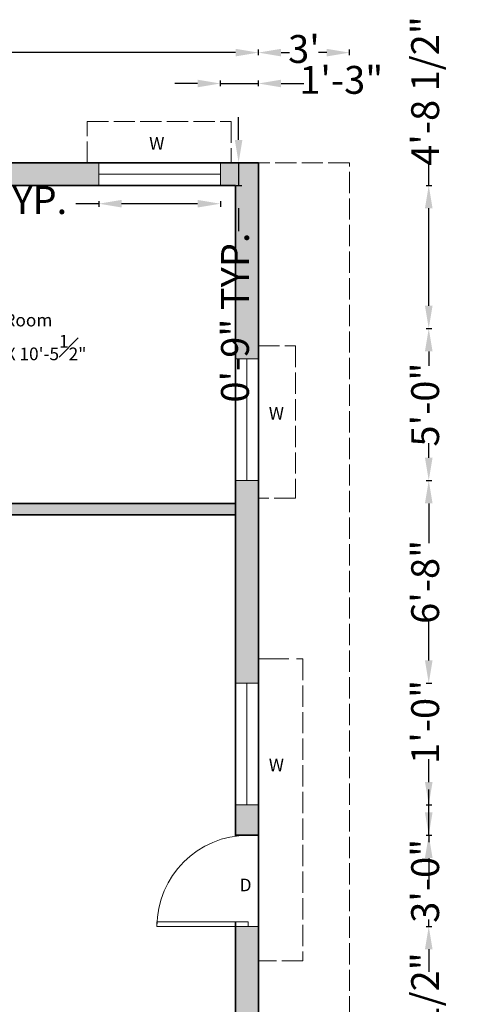
# Model space of a CAD drawing. Units: inches. Extents: x 2339 to 2848, y 489 to 1121.
# Tile 3 of 3: x 2670 to 2848, y 725 to 1114. Entities that reach past the tile are written whole.
import ezdxf

# ---------------------------------------------------------------- set-up
doc = ezdxf.new("R2010")
doc.units = ezdxf.units.IN
doc.linetypes.add('ACAD_ISO02W100', pattern=[15, 12, -3])
for name, color, linetype, lineweight in [('A-ANNO-DIMS', 2, 'Continuous', 18), ('A-ANNO-TEXT', 7, 'Continuous', 18), ('A-AREA-IDEN', 7, 'Continuous', 18), ('A-DOOR', 3, 'Continuous', 18), ('A-GLAZ', 4, 'Continuous', 18), ('A-ROOF-OVHD', 8, 'ACAD_ISO02W100', 13), ('A-WALL', 7, 'Continuous', 35), ('C-PROP', 8, 'ACAD_ISO02W100', 18)]:
    doc.layers.add(name, color=color, linetype=linetype, lineweight=lineweight)
doc.layers.add('A-WALL-PATT', color=18, linetype='Continuous', lineweight=13, true_color=0x000000)
doc.styles.get("Standard").update_dxf_attribs({"font": 'arial.ttf'})
doc.dimstyles.new('ISO-25', dxfattribs={"dimtxt": 11, "dimasz": 9, "dimexe": 1.25, "dimexo": 0.625, "dimtad": 0, "dimlunit": 4, "dimtxsty": 'Standard', "dimcen": 2.5, "dimadec": 0, "dimazin": 0, "dimtfac": 1, "dimtmove": 0, "dimatfit": 3, "dimfxl": 1, "dimfxlon": 1, "dimfrac": 1, "dimarcsym": 0})

# ---------------------------------------------------------------- blocks, each defined once
blk = doc.blocks.new('*U2')
for p, q in [((0, 0), (0, -4)), ((36, 0), (36, -4))]:
    blk.add_line(p, q)
blk.add_lwpolyline([(0, 0), (0, 36), (1.75, 36), (1.75, 0)], close=True)
blk.add_arc((0, 0), 36, 0, 90)
blk = doc.blocks.new('*D6')
at = {"layer": 'A-ANNO-DIMS', "color": 0, "lineweight": -2, "transparency": 16777216}
for p, q in [((2402.35, 1099.88), (2402.35, 1102.13)), ((2411.35, 1100.88), (2563.83, 1100.88)), ((2755.35, 1100.88), (2602.86, 1100.88)), ((2764.35, 1099.88), (2764.35, 1102.13))]:
    blk.add_line(p, q, dxfattribs=at)
at = {"layer": 'A-ANNO-DIMS', "color": 0, "transparency": 16777216}
for points in [[(2411.35, 1102.38), (2411.35, 1099.38), (2402.35, 1100.88)], [(2755.35, 1102.38), (2755.35, 1099.38), (2764.35, 1100.88)]]:
    blk.add_solid(points, dxfattribs=at)
at = {"layer": 'Defpoints', "color": 0, "transparency": 16777216}
for p in [(2764.35, 1100.88), (2402.35, 1057.44), (2764.35, 1057.44)]:
    blk.add_point(p, dxfattribs=at)
at = {"layer": 'A-ANNO-DIMS', "color": 0, "transparency": 16777216, "insert": (2583.35, 1100.88), "char_height": 11, "attachment_point": 5}
blk.add_mtext('30\'-2"', dxfattribs=at)
blk = doc.blocks.new('*D7')
at = {"layer": 'A-ANNO-DIMS', "color": 0, "lineweight": -2, "transparency": 16777216}
for p, q in [((2764.35, 1099.88), (2764.35, 1102.13)), ((2773.35, 1100.88), (2776.66, 1100.88)), ((2791.35, 1100.88), (2788.03, 1100.88)), ((2800.35, 1099.88), (2800.35, 1102.13))]:
    blk.add_line(p, q, dxfattribs=at)
at = {"layer": 'A-ANNO-DIMS', "color": 0, "transparency": 16777216}
for points in [[(2773.35, 1102.38), (2773.35, 1099.38), (2764.35, 1100.88)], [(2791.35, 1102.38), (2791.35, 1099.38), (2800.35, 1100.88)]]:
    blk.add_solid(points, dxfattribs=at)
at = {"layer": 'Defpoints', "color": 0, "transparency": 16777216}
for p in [(2800.35, 1100.88), (2764.35, 1057.44), (2800.35, 1057.44)]:
    blk.add_point(p, dxfattribs=at)
at = {"layer": 'A-ANNO-DIMS', "color": 0, "transparency": 16777216, "insert": (2782.35, 1100.88), "char_height": 11, "attachment_point": 5}
blk.add_mtext("3'", dxfattribs=at)
blk = doc.blocks.new('WIN-48IN')
for p, q in [((0, 0), (0, 9)), ((48, 0), (48, 9)), ((0, 4.5), (48, 4.5))]:
    blk.add_line(p, q)
blk = doc.blocks.new('*D9')
at = {"layer": 'A-ANNO-DIMS', "color": 0, "lineweight": -2, "transparency": 16777216}
for p, q in [((2701.35, 1042.24), (2701.35, 1039.99)), ((2749.35, 1042.24), (2749.35, 1039.99)), ((2701.35, 1041.24), (2692.35, 1041.24)), ((2740.35, 1041.24), (2710.35, 1041.24))]:
    blk.add_line(p, q, dxfattribs=at)
at = {"layer": 'A-ANNO-DIMS', "color": 0, "transparency": 16777216}
for points in [[(2710.35, 1042.74), (2710.35, 1039.74), (2701.35, 1041.24)], [(2740.35, 1042.74), (2740.35, 1039.74), (2749.35, 1041.24)]]:
    blk.add_solid(points, dxfattribs=at)
at = {"layer": 'Defpoints', "color": 0, "transparency": 16777216}
for p in [(2701.35, 1048.44), (2749.35, 1048.44), (2701.35, 1041.24)]:
    blk.add_point(p, dxfattribs=at)
at = {"layer": 'A-ANNO-DIMS', "color": 0, "transparency": 16777216, "insert": (2622.12, 1041.24), "char_height": 11, "attachment_point": 5}
blk.add_mtext('WINDOW 4\'-0" TYP.', dxfattribs=at)
blk = doc.blocks.new('*D10')
at = {"layer": 'A-ANNO-DIMS', "color": 0, "lineweight": -2, "transparency": 16777216}
for p, q in [((2756.55, 1066.44), (2756.55, 1075.44)), ((2755.55, 1057.44), (2757.8, 1057.44)), ((2756.55, 1057.44), (2756.55, 1048.44)), ((2755.55, 1048.44), (2757.8, 1048.44)), ((2756.55, 1039.44), (2756.55, 1030.44))]:
    blk.add_line(p, q, dxfattribs=at)
at = {"layer": 'A-ANNO-DIMS', "color": 0, "transparency": 16777216}
for points in [[(2755.05, 1066.44), (2758.05, 1066.44), (2756.55, 1057.44)], [(2755.05, 1039.44), (2758.05, 1039.44), (2756.55, 1048.44)]]:
    blk.add_solid(points, dxfattribs=at)
at = {"layer": 'Defpoints', "color": 0, "transparency": 16777216}
for p in [(2749.35, 1057.44), (2749.35, 1048.44), (2756.55, 1048.44)]:
    blk.add_point(p, dxfattribs=at)
at = {"layer": 'A-ANNO-DIMS', "color": 0, "transparency": 16777216, "insert": (2756.55, 996.29), "char_height": 11, "attachment_point": 5, "rotation": 90}
blk.add_mtext('0\'-9" TYP.', dxfattribs=at)
blk = doc.blocks.new('*D25')
at = {"layer": 'A-ANNO-DIMS', "color": 0, "lineweight": -2, "transparency": 16777216}
for p, q in [((2830.6, 991.94), (2832.85, 991.94)), ((2831.6, 982.94), (2831.6, 977.18)), ((2831.6, 940.94), (2831.6, 946.69)), ((2830.6, 931.94), (2832.85, 931.94))]:
    blk.add_line(p, q, dxfattribs=at)
at = {"layer": 'A-ANNO-DIMS', "color": 0, "transparency": 16777216}
for points in [[(2830.1, 982.94), (2833.1, 982.94), (2831.6, 991.94)], [(2830.1, 940.94), (2833.1, 940.94), (2831.6, 931.94)]]:
    blk.add_solid(points, dxfattribs=at)
at = {"layer": 'Defpoints', "color": 0, "transparency": 16777216}
for p in [(2411.35, 991.94), (2831.6, 991.94), (2411.35, 931.94)]:
    blk.add_point(p, dxfattribs=at)
at = {"layer": 'A-ANNO-DIMS', "color": 0, "transparency": 16777216, "insert": (2831.6, 961.94), "char_height": 11, "attachment_point": 5, "rotation": 90}
blk.add_mtext('5\'-0"', dxfattribs=at)
blk = doc.blocks.new('*D26')
at = {"layer": 'A-ANNO-DIMS', "color": 0, "lineweight": -2, "transparency": 16777216}
for p, q in [((2831.6, 1048.44), (2831.6, 1057.44)), ((2830.6, 1048.44), (2832.85, 1048.44)), ((2831.6, 1000.94), (2831.6, 1039.44)), ((2830.6, 991.94), (2832.85, 991.94))]:
    blk.add_line(p, q, dxfattribs=at)
at = {"layer": 'A-ANNO-DIMS', "color": 0, "transparency": 16777216}
for points in [[(2830.1, 1039.44), (2833.1, 1039.44), (2831.6, 1048.44)], [(2830.1, 1000.94), (2833.1, 1000.94), (2831.6, 991.94)]]:
    blk.add_solid(points, dxfattribs=at)
at = {"layer": 'Defpoints', "color": 0, "transparency": 16777216}
for p in [(2411.35, 1048.44), (2831.6, 1048.44), (2411.35, 991.94)]:
    blk.add_point(p, dxfattribs=at)
at = {"layer": 'A-ANNO-DIMS', "color": 0, "transparency": 16777216, "insert": (2831.6, 1085.72), "char_height": 11, "attachment_point": 5, "rotation": 90}
blk.add_mtext('4\'-8 1/2"', dxfattribs=at)
blk = doc.blocks.new('*D30')
at = {"layer": 'A-ANNO-DIMS', "color": 0, "lineweight": -2, "transparency": 16777216}
for p, q in [((2740.35, 1088.69), (2731.35, 1088.69)), ((2749.35, 1087.69), (2749.35, 1089.94)), ((2749.35, 1088.69), (2764.35, 1088.69)), ((2764.35, 1087.69), (2764.35, 1089.94)), ((2773.35, 1088.69), (2782.35, 1088.69))]:
    blk.add_line(p, q, dxfattribs=at)
at = {"layer": 'A-ANNO-DIMS', "color": 0, "transparency": 16777216}
for points in [[(2740.35, 1090.19), (2740.35, 1087.19), (2749.35, 1088.69)], [(2773.35, 1090.19), (2773.35, 1087.19), (2764.35, 1088.69)]]:
    blk.add_solid(points, dxfattribs=at)
at = {"layer": 'Defpoints', "color": 0, "transparency": 16777216}
for p in [(2764.35, 1088.69), (2749.35, 1057.44), (2764.35, 1057.44)]:
    blk.add_point(p, dxfattribs=at)
at = {"layer": 'A-ANNO-DIMS', "color": 0, "transparency": 16777216, "insert": (2797.07, 1088.69), "char_height": 11, "attachment_point": 5}
blk.add_mtext('1\'-3"', dxfattribs=at)
blk = doc.blocks.new('*D32')
at = {"layer": 'A-ANNO-DIMS', "color": 0, "lineweight": -2, "transparency": 16777216}
for p, q in [((2830.6, 755.94), (2832.85, 755.94)), ((2831.6, 746.94), (2831.6, 744.28)), ((2831.6, 685.44), (2831.6, 688.1)), ((2830.6, 676.44), (2832.85, 676.44))]:
    blk.add_line(p, q, dxfattribs=at)
at = {"layer": 'A-ANNO-DIMS', "color": 0, "transparency": 16777216}
for points in [[(2830.1, 746.94), (2833.1, 746.94), (2831.6, 755.94)], [(2830.1, 685.44), (2833.1, 685.44), (2831.6, 676.44)]]:
    blk.add_solid(points, dxfattribs=at)
at = {"layer": 'Defpoints', "color": 0, "transparency": 16777216}
for p in [(2764.35, 755.94), (2831.6, 755.94), (2764.35, 676.44)]:
    blk.add_point(p, dxfattribs=at)
at = {"layer": 'A-ANNO-DIMS', "color": 0, "transparency": 16777216, "insert": (2831.6, 716.19), "char_height": 11, "attachment_point": 5, "rotation": 90}
blk.add_mtext('6\'-7 1/2"', dxfattribs=at)
blk = doc.blocks.new('*D33')
at = {"layer": 'A-ANNO-DIMS', "color": 0, "lineweight": -2, "transparency": 16777216}
for p, q in [((2831.6, 800.94), (2831.6, 809.94)), ((2830.6, 791.94), (2832.85, 791.94)), ((2831.6, 791.94), (2831.6, 789.18)), ((2831.6, 755.94), (2831.6, 758.7)), ((2830.6, 755.94), (2832.85, 755.94)), ((2831.6, 746.94), (2831.6, 737.94))]:
    blk.add_line(p, q, dxfattribs=at)
at = {"layer": 'A-ANNO-DIMS', "color": 0, "transparency": 16777216}
for points in [[(2830.1, 800.94), (2833.1, 800.94), (2831.6, 791.94)], [(2830.1, 746.94), (2833.1, 746.94), (2831.6, 755.94)]]:
    blk.add_solid(points, dxfattribs=at)
at = {"layer": 'Defpoints', "color": 0, "transparency": 16777216}
for p in [(2764.35, 791.94), (2831.6, 791.94), (2764.35, 755.94)]:
    blk.add_point(p, dxfattribs=at)
at = {"layer": 'A-ANNO-DIMS', "color": 0, "transparency": 16777216, "insert": (2831.6, 773.94), "char_height": 11, "attachment_point": 5, "rotation": 90}
blk.add_mtext('3\'-0"', dxfattribs=at)
blk = doc.blocks.new('*D34')
at = {"layer": 'A-ANNO-DIMS', "color": 0, "lineweight": -2, "transparency": 16777216}
for p, q in [((2831.6, 812.94), (2831.6, 821.94)), ((2830.6, 803.94), (2832.85, 803.94)), ((2831.6, 791.94), (2831.6, 803.94)), ((2830.6, 791.94), (2832.85, 791.94)), ((2831.6, 782.94), (2831.6, 773.94))]:
    blk.add_line(p, q, dxfattribs=at)
at = {"layer": 'A-ANNO-DIMS', "color": 0, "transparency": 16777216}
for points in [[(2830.1, 812.94), (2833.1, 812.94), (2831.6, 803.94)], [(2830.1, 782.94), (2833.1, 782.94), (2831.6, 791.94)]]:
    blk.add_solid(points, dxfattribs=at)
at = {"layer": 'Defpoints', "color": 0, "transparency": 16777216}
for p in [(2764.35, 803.94), (2831.6, 803.94), (2764.35, 791.94)]:
    blk.add_point(p, dxfattribs=at)
at = {"layer": 'A-ANNO-DIMS', "color": 0, "transparency": 16777216, "insert": (2831.6, 836.67), "char_height": 11, "attachment_point": 5, "rotation": 90}
blk.add_mtext('1\'-0"', dxfattribs=at)
blk = doc.blocks.new('*D35')
at = {"layer": 'A-ANNO-DIMS', "color": 0, "lineweight": -2, "transparency": 16777216}
for p, q in [((2830.6, 931.94), (2832.85, 931.94)), ((2831.6, 922.94), (2831.6, 907.21)), ((2831.6, 860.94), (2831.6, 876.66)), ((2830.6, 851.94), (2832.85, 851.94))]:
    blk.add_line(p, q, dxfattribs=at)
at = {"layer": 'A-ANNO-DIMS', "color": 0, "transparency": 16777216}
for points in [[(2830.1, 922.94), (2833.1, 922.94), (2831.6, 931.94)], [(2830.1, 860.94), (2833.1, 860.94), (2831.6, 851.94)]]:
    blk.add_solid(points, dxfattribs=at)
at = {"layer": 'Defpoints', "color": 0, "transparency": 16777216}
for p in [(2764.35, 931.94), (2831.6, 931.94), (2764.35, 851.94)]:
    blk.add_point(p, dxfattribs=at)
at = {"layer": 'A-ANNO-DIMS', "color": 0, "transparency": 16777216, "insert": (2831.6, 891.94), "char_height": 11, "attachment_point": 5, "rotation": 90}
blk.add_mtext('6\'-8"', dxfattribs=at)

msp = doc.modelspace()

# ---------------------------------------------------------------- hatches: boundary and pattern name
at = {"layer": 'A-WALL-PATT'}
h = msp.add_hatch(color=256, dxfattribs=at)
h.dxf.hatch_style = 1
h.paths.add_polyline_path([(2493.847, 1057.438), (2402.347, 1057.438), (2402.347, 991.938), (2411.347, 991.938), (2411.347, 1048.438), (2493.847, 1048.438)])
h.paths.add_polyline_path([(2411.347, 931.938), (2402.347, 931.938), (2402.347, 912.438), (2411.347, 912.438), (2411.347, 918.438)])
h.paths.add_polyline_path([(2411.347, 871.438), (2411.347, 877.438), (2402.347, 877.438), (2402.347, 803.938), (2411.347, 803.938)])
h.paths.add_polyline_path([(2547.847, 871.438), (2411.347, 871.438), (2411.347, 866.938), (2547.847, 866.938)])
h.paths.add_polyline_path([(2447.347, 922.938), (2411.347, 922.938), (2411.347, 918.438), (2447.347, 918.438)])
h.paths.add_polyline_path([(2552.347, 866.938), (2547.847, 866.938), (2547.847, 791.938), (2552.347, 791.938)])
h.paths.add_polyline_path([(2411.347, 755.938), (2402.347, 755.938), (2402.347, 670.438), (2411.347, 670.438)])
h.paths.add_polyline_path([(2552.347, 755.938), (2547.847, 755.938), (2547.847, 746.938), (2411.347, 746.938), (2411.347, 742.438), (2547.847, 742.438), (2547.847, 737.938), (2552.347, 737.938)])
h.paths.add_polyline_path([(2552.347, 701.938), (2547.847, 701.938), (2547.847, 622.438), (2552.347, 622.438)])
h.paths.add_polyline_path([(2581.347, 622.438), (2411.347, 622.438), (2411.347, 634.438), (2402.347, 634.438), (2402.347, 613.438), (2581.347, 613.438)])
h.paths.add_polyline_path([(2695.347, 622.438), (2635.347, 622.438), (2635.347, 613.438), (2695.347, 613.438)])
h.paths.add_polyline_path([(2764.347, 628.438), (2755.347, 628.438), (2755.347, 622.438), (2749.347, 622.438), (2749.347, 613.438), (2764.347, 613.438)])
h.paths.add_polyline_path([(2764.347, 755.938), (2760.347, 755.938), (2755.347, 755.938), (2755.347, 676.438), (2764.347, 676.438)])
h.paths.add_polyline_path([(2764.347, 931.938), (2755.347, 931.938), (2755.347, 851.938), (2764.347, 851.938)])
h.paths.add_polyline_path([(2764.347, 1057.438), (2749.347, 1057.438), (2749.347, 1048.438), (2755.347, 1048.438), (2755.347, 979.938), (2764.347, 979.938)])
h.paths.add_polyline_path([(2701.347, 1057.438), (2594.347, 1057.438), (2594.347, 1048.438), (2604.847, 1048.438), (2701.347, 1048.438)])
h.paths.add_polyline_path([(2558.347, 1057.438), (2541.847, 1057.438), (2541.847, 1048.438), (2552.347, 1048.438), (2558.347, 1048.438)])
h = msp.add_hatch(color=256, dxfattribs=at)
h.dxf.hatch_style = 1
h.paths.add_polyline_path([(2552.347, 1048.438), (2547.847, 1048.438), (2547.847, 967.438), (2551.847, 967.438), (2552.347, 967.438), (2552.347, 971.938), (2563.847, 971.938), (2563.847, 976.438), (2552.347, 976.438)])
h.paths.add_polyline_path([(2604.847, 1048.438), (2600.347, 1048.438), (2600.347, 976.438), (2595.847, 976.438), (2595.847, 972.438), (2595.847, 971.938), (2600.347, 971.938), (2600.347, 967.438), (2604.347, 967.438, -0.0034723), (2604.847, 967.434)])
h.paths.add_polyline_path([(2604.847, 922.938), (2604.847, 931.438), (2604.347, 931.438), (2600.347, 931.438), (2600.347, 918.438), (2755.347, 918.438), (2755.347, 922.938)])
h = msp.add_hatch(color=256, dxfattribs=at)
h.dxf.hatch_style = 1
h.paths.add_polyline_path([(2764.347, 803.938), (2755.347, 803.938), (2755.347, 791.938), (2764.347, 791.938)])

# ---------------------------------------------------------------- linework, layer by layer
at = {"layer": 'A-ROOF-OVHD', "ltscale": 0.7}
for p, q in [((2696.763, 1057.438), (2696.763, 1073.72)), ((2696.763, 1073.72), (2753.635, 1073.72)), ((2753.635, 1073.72), (2753.635, 1057.438)), ((2764.347, 985.073), (2778.997, 985.073)), ((2778.997, 985.073), (2778.997, 925.042)), ((2778.997, 925.042), (2764.347, 925.042)), ((2781.956, 861.575), (2781.956, 742.291)), ((2781.956, 742.291), (2764.347, 742.291))]:
    msp.add_line(p, q, dxfattribs=at)
at = {"layer": 'A-ROOF-OVHD'}
msp.add_line((2764.347, 861.575), (2781.956, 861.575), dxfattribs=at)
at = {"layer": 'A-WALL'}
for p, q in [((2764.347, 1057.438), (2402.347, 1057.438)), ((2764.347, 791.938), (2764.347, 1057.438)), ((2755.347, 1048.438), (2604.847, 1048.438)), ((2755.347, 791.589), (2755.347, 1048.438)), ((2755.347, 922.938), (2604.847, 922.938)), ((2755.347, 918.438), (2600.347, 918.438)), ((2764.347, 791.938), (2755.347, 791.938)), ((2764.347, 613.438), (2764.347, 791.938)), ((2755.347, 622.438), (2755.347, 757.688))]:
    msp.add_line(p, q, dxfattribs=at)
at = {"layer": 'C-PROP', "ltscale": 0.7}
for p, q in [((2800.347, 1057.438), (2764.347, 1057.438)), ((2800.347, 541.438), (2800.347, 1057.438))]:
    msp.add_line(p, q, dxfattribs=at)

# ---------------------------------------------------------------- block references
at = {"layer": 'A-DOOR', "rotation": 90}
msp.add_blockref('*U2', (2760.347, 755.938), dxfattribs=at)
at = {"layer": 'A-GLAZ'}
for p, rotation in [((2749.347, 1057.438), 180), ((2755.347, 979.938), 269.9999999999995), ((2755.347, 851.938), 269.9999999999995)]:
    msp.add_blockref('WIN-48IN', p, dxfattribs=dict(at, rotation=rotation))

# ---------------------------------------------------------------- texts
at = {"layer": 'A-ANNO-TEXT', "ltscale": 0.7, "char_height": 5, "attachment_point": 1}
for insert in [(2717.154, 1067.51), (2764.347, 961.003), (2764.347, 822.18)]:
    msp.add_mtext_dynamic_manual_height_columns('\\pxqc;W', width=14.23587, gutter_width=12.5, heights=[0], dxfattribs=dict(at, insert=insert))
at = {"layer": 'A-ANNO-TEXT', "insert": (2752.198, 774.797), "char_height": 5, "attachment_point": 1}
msp.add_mtext_dynamic_manual_height_columns('\\pxqc;D', width=14.23587, gutter_width=12.5, heights=[0], dxfattribs=at)
at = {"layer": 'A-AREA-IDEN', "insert": (2617.965, 997.789), "char_height": 5, "attachment_point": 1}
msp.add_mtext_dynamic_manual_height_columns('\\pxqc;Bed Room\\P12\'-6\\S1#2;" X 10\'-5\\S1#2;"', width=97.24493, gutter_width=12.5, heights=[0], dxfattribs=at)

# ---------------------------------------------------------------- dimensions: what is measured, and where the dimension line sits
at = {"layer": 'A-ANNO-DIMS'}
for base, p1, p2, angle, picture, middle in [((2831.597, 1048.438), (2411.347, 991.938), (2411.347, 1048.438), 90, '*D26', (2831.597, 1085.72)), ((2764.347, 1088.688), (2749.347, 1057.438), (2764.347, 1057.438), 0, '*D30', (2797.074, 1088.688)), ((2831.597, 991.938), (2411.347, 931.938), (2411.347, 991.938), 90, '*D25', (2831.597, 961.938)), ((2831.597, 931.938), (2764.347, 851.938), (2764.347, 931.938), 90, '*D35', (2831.597, 891.938)), ((2831.597, 803.938), (2764.347, 791.938), (2764.347, 803.938), 90, '*D34', (2831.597, 836.665)), ((2831.597, 791.938), (2764.347, 755.938), (2764.347, 791.938), 90, '*D33', (2831.597, 773.938)), ((2831.597, 755.938), (2764.347, 676.438), (2764.347, 755.938), 90, '*D32', (2831.597, 716.188))]:
    dim = msp.add_linear_dim(base=base, p1=p1, p2=p2, angle=angle, dimstyle='ISO-25', override={"dimdec": 1, "dimlfac": 1, "dimrnd": 0, "dimzin": 1, "dimdsep": 46, "dimlunit": 4, "dimfrac": 2}, dxfattribs=at)
    dim.commit()
    dim.dimension.update_dxf_attribs({"geometry": picture, "text_midpoint": middle})
for base, p1, p2, override, picture, middle in [((2764.347, 1100.878), (2402.347, 1057.438), (2764.347, 1057.438), {"dimclrd": 0, "dimclre": 0, "dimclrt": 0}, '*D6', (2583.347, 1100.878)), ((2800.347, 1100.878), (2764.347, 1057.438), (2800.347, 1057.438), {"dimclrd": 0, "dimclre": 0, "dimclrt": 0, "dimtmove": 1}, '*D7', (2782.347, 1100.878))]:
    dim = msp.add_linear_dim(base=base, p1=p1, p2=p2, dimstyle='ISO-25', override=override, dxfattribs=at)
    dim.commit()
    dim.dimension.update_dxf_attribs({"geometry": picture, "text_midpoint": middle})
for base, p1, p2, angle, text, picture, middle in [((2756.547, 1048.438), (2749.347, 1057.438), (2749.347, 1048.438), 270, '<> TYP.', '*D10', (2756.547, 996.287)), ((2701.347, 1041.238), (2749.347, 1048.438), (2701.347, 1048.438), 180, 'WINDOW <> TYP.', '*D9', (2622.124, 1041.238))]:
    dim = msp.add_linear_dim(base=base, p1=p1, p2=p2, angle=angle, text=text, dimstyle='ISO-25', override={"dimdec": 1, "dimlfac": 1, "dimrnd": 0, "dimzin": 1, "dimdsep": 46, "dimlunit": 4, "dimfrac": 2}, dxfattribs=at)
    dim.commit()
    dim.dimension.update_dxf_attribs({"geometry": picture, "text_midpoint": middle})

doc.saveas('drawing.dxf')
